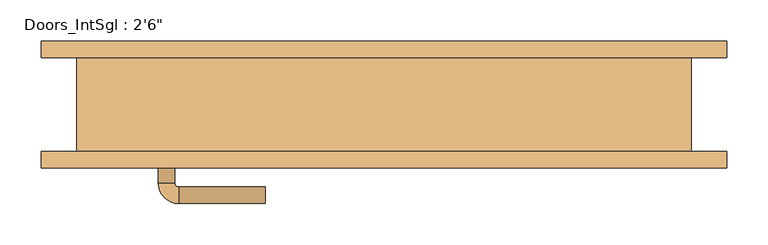
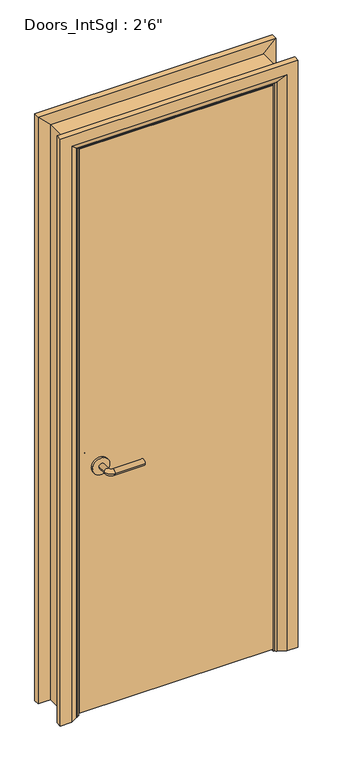
"""IFC4 building model written with IfcOpenShell, lengths in millimetres: door geometry."""

from ifc_helpers import new_model, si_unit, point, frame, frame_2d, origin, place, context, project, spatial, polyline, circle_curve, ellipse_curve, trimmed, segment, composite_curve, outline, extrude, faceted_brep, source, transform, mapped, element, save
from ifc_brep_helpers import plane_surface, cylinder_surface, revolved_surface, advanced_brep


def door_d225582b(model_context):
    return source(origin(), model_context, "Body", "SolidModel", [
        advanced_brep(
        [(-274.0, -11.15, 900.0), (-254.0, -11.15, 900.0), (-274.0, 18.85, 900.0), (-254.0, 18.85, 900.0), (-249.0, 23.85, 900.0), (-249.0, 43.85, 900.0), (-144.0, 43.85, 900.0), (-144.0, 23.85, 900.0)],
        [
            (0, 1, circle_curve(frame((-264.0, -11.15, 900.0), z_axis=(0.0, -1.0, 0.0), x_axis=(1.0, 0.0, 0.0)), 10.0)),
            (1, 0, circle_curve(frame((-264.0, -11.15, 900.0), z_axis=(0.0, -1.0, 0.0), x_axis=(1.0, 0.0, 0.0)), 10.0)),
            (0, 2),
            (2, 3, circle_curve(frame((-264.0, 18.85, 900.0), z_axis=(0.0, -1.0, 0.0), x_axis=(1.0, 0.0, 0.0)), 10.0)),
            (3, 1),
            (3, 2, circle_curve(frame((-264.0, 18.85, 900.0), z_axis=(0.0, -1.0, 0.0), x_axis=(1.0, 0.0, 0.0)), 10.0)),
            (4, 3, circle_curve(frame((-249.0, 18.85, 900.0), z_axis=(0.0, 0.0, 1.0), x_axis=(-1.0, 0.0, 0.0)), 5.0)),
            (2, 5, circle_curve(frame((-249.0, 18.85, 900.0), z_axis=(0.0, 0.0, -1.0), x_axis=(-1.0, 0.0, 0.0)), 25.0)),
            (5, 4, circle_curve(frame((-249.0, 33.85, 900.0), z_axis=(-1.0, 0.0, 0.0), x_axis=(0.0, -1.0, 0.0)), 10.0)),
            (4, 5, circle_curve(frame((-249.0, 33.85, 900.0), z_axis=(-1.0, 0.0, 0.0), x_axis=(0.0, -1.0, 0.0)), 10.0)),
            (6, 7, circle_curve(frame((-144.0, 33.85, 900.0), z_axis=(1.0, 0.0, 0.0), x_axis=(0.0, -1.0, 0.0)), 10.0)),
            (7, 6, circle_curve(frame((-144.0, 33.85, 900.0), z_axis=(1.0, 0.0, 0.0), x_axis=(0.0, -1.0, 0.0)), 10.0)),
            (5, 6),
            (7, 4),
        ],
        [
            plane_surface(frame((-264.0, -11.15, 900.0), z_axis=(0.0, -1.0, 0.0), x_axis=(0.0, 0.0, 1.0))),
            cylinder_surface(frame((-264.0, -11.15, 900.0), z_axis=(0.0, -1.0, 0.0), x_axis=(1.0, 0.0, 0.0)), 10.0),
            revolved_surface(trimmed(ellipse_curve(frame((-264.0, 18.85, 900.0), z_axis=(0.0, -1.0, 0.0), x_axis=(1.0, 0.0, 0.0)), 10.0, 10.0), [point((-274.0, 18.85, 900.0))], [point((-254.0, 18.85, 900.0))], True, "CARTESIAN"), (-249.0, 18.85, 900.0), (0.0, 0.0, -1.0)),
            revolved_surface(trimmed(ellipse_curve(frame((-264.0, 18.85, 900.0), z_axis=(0.0, -1.0, 0.0), x_axis=(1.0, 0.0, 0.0)), 10.0, 10.0), [point((-254.0, 18.85, 900.0))], [point((-274.0, 18.85, 900.0))], True, "CARTESIAN"), (-249.0, 18.85, 900.0), (0.0, 0.0, -1.0)),
            plane_surface(frame((-144.0, 33.85, 900.0), z_axis=(1.0, 0.0, 0.0), x_axis=(0.0, 0.0, 1.0))),
            cylinder_surface(frame((-249.0, 33.85, 900.0), z_axis=(-1.0, 0.0, 0.0), x_axis=(0.0, -1.0, 0.0)), 10.0),
        ],
        [
            (0, [[1, 2]]),
            (1, [[-1, 3, 4, 5]]),
            (1, [[-2, -5, 6, -3]]),
            (2, [[7, -4, 8, 9]]),
            (3, [[-8, -6, -7, 10]]),
            (4, [[11, 12]]),
            (5, [[-9, 13, -12, 14]]),
            (5, [[-10, -14, -11, -13]]),
        ],
    ),
        extrude(outline(composite_curve([segment(trimmed(circle_curve(frame_2d((900.0, -266.5)), 30.0), [point((900.0, -296.5))], [point((900.0, -236.5))], False, "CARTESIAN"), True, "CONTINUOUS"), segment(trimmed(circle_curve(frame_2d((900.0, -266.5)), 30.0), [point((900.0, -236.5))], [point((900.0, -296.5))], False, "CARTESIAN"), True, "CONTINUOUS")], self_intersect=False)), frame((0.0, -19.15, 0.0), z_axis=(0.0, 1.0, 0.0), x_axis=(0.0, 0.0, 1.0)), (0.0, 0.0, 1.0), 8.0),
        advanced_brep(
        [(-274.0, -65.15, 900.0), (-254.0, -65.15, 900.0), (-254.0, -95.15, 900.0), (-274.0, -95.15, 900.0), (-249.0, -100.15, 900.0), (-249.0, -120.15, 900.0), (-144.0, -120.15, 900.0), (-144.0, -100.15, 900.0)],
        [
            (0, 1, circle_curve(frame((-264.0, -65.15, 900.0), z_axis=(0.0, 1.0, 0.0), x_axis=(1.0, 0.0, 0.0)), 10.0)),
            (1, 0, circle_curve(frame((-264.0, -65.15, 900.0), z_axis=(0.0, 1.0, 0.0), x_axis=(1.0, 0.0, 0.0)), 10.0)),
            (1, 2),
            (2, 3, circle_curve(frame((-264.0, -95.15, 900.0), z_axis=(0.0, 1.0, 0.0), x_axis=(1.0, 0.0, 0.0)), 10.0)),
            (3, 0),
            (3, 2, circle_curve(frame((-264.0, -95.15, 900.0), z_axis=(0.0, 1.0, 0.0), x_axis=(1.0, 0.0, 0.0)), 10.0)),
            (4, 5, circle_curve(frame((-249.0, -110.15, 900.0), z_axis=(-1.0, 0.0, 0.0), x_axis=(0.0, 1.0, 0.0)), 10.0)),
            (5, 3, circle_curve(frame((-249.0, -95.15, 900.0), z_axis=(0.0, 0.0, -1.0), x_axis=(-1.0, 0.0, 0.0)), 25.0)),
            (2, 4, circle_curve(frame((-249.0, -95.15, 900.0), z_axis=(0.0, 0.0, 1.0), x_axis=(-1.0, 0.0, 0.0)), 5.0)),
            (5, 4, circle_curve(frame((-249.0, -110.15, 900.0), z_axis=(-1.0, 0.0, 0.0), x_axis=(0.0, 1.0, 0.0)), 10.0)),
            (6, 7, circle_curve(frame((-144.0, -110.15, 900.0), z_axis=(1.0, 0.0, 0.0), x_axis=(0.0, 1.0, 0.0)), 10.0)),
            (7, 6, circle_curve(frame((-144.0, -110.15, 900.0), z_axis=(1.0, 0.0, 0.0), x_axis=(0.0, 1.0, 0.0)), 10.0)),
            (4, 7),
            (6, 5),
        ],
        [
            plane_surface(frame((-264.0, -65.15, 900.0), z_axis=(0.0, 1.0, 0.0), x_axis=(0.0, 0.0, 1.0))),
            cylinder_surface(frame((-264.0, -65.15, 900.0), z_axis=(0.0, 1.0, 0.0), x_axis=(1.0, 0.0, 0.0)), 10.0),
            revolved_surface(trimmed(ellipse_curve(frame((-264.0, -95.15, 900.0), z_axis=(0.0, -1.0, 0.0), x_axis=(1.0, 0.0, 0.0)), 10.0, 10.0), [point((-274.0, -95.15, 900.0))], [point((-254.0, -95.15, 900.0))], True, "CARTESIAN"), (-249.0, -95.15, 900.0), (0.0, 0.0, -1.0)),
            revolved_surface(trimmed(ellipse_curve(frame((-264.0, -95.15, 900.0), z_axis=(0.0, -1.0, 0.0), x_axis=(1.0, 0.0, 0.0)), 10.0, 10.0), [point((-254.0, -95.15, 900.0))], [point((-274.0, -95.15, 900.0))], True, "CARTESIAN"), (-249.0, -95.15, 900.0), (0.0, 0.0, -1.0)),
            plane_surface(frame((-144.0, -110.15, 900.0), z_axis=(1.0, 0.0, 0.0), x_axis=(0.0, 0.0, 1.0))),
            cylinder_surface(frame((-249.0, -110.15, 900.0), z_axis=(-1.0, 0.0, 0.0), x_axis=(0.0, 1.0, 0.0)), 10.0),
        ],
        [
            (0, [[1, 2]]),
            (1, [[3, 4, 5, -2]]),
            (1, [[-5, 6, -3, -1]]),
            (2, [[7, 8, -4, 9]]),
            (3, [[10, -9, -6, -8]]),
            (4, [[11, 12]]),
            (5, [[13, -11, 14, -7]]),
            (5, [[-14, -12, -13, -10]]),
        ],
    ),
        extrude(outline(composite_curve([segment(trimmed(circle_curve(frame_2d((900.0, -266.5)), 30.0), [point((900.0, -296.5))], [point((900.0, -236.5))], False, "CARTESIAN"), True, "CONTINUOUS"), segment(trimmed(circle_curve(frame_2d((900.0, -266.5)), 30.0), [point((900.0, -236.5))], [point((900.0, -296.5))], False, "CARTESIAN"), True, "CONTINUOUS")], self_intersect=False)), frame((0.0, -65.15, 0.0), z_axis=(0.0, 1.0, 0.0), x_axis=(0.0, 0.0, 1.0)), (0.0, 0.0, 1.0), 8.0),
        extrude(outline(polyline([(339.0, -19.15), (339.0, -57.15), (-339.0, -57.15), (-339.0, -19.15), (339.0, -19.15)])), frame((0.0, 0.0, 8.0), z_axis=(0.0, 0.0, 1.0), x_axis=(1.0, 0.0, 0.0)), (0.0, 0.0, 1.0), 2083.6),
        advanced_brep(
        [(416.0, -77.15, 0.0), (376.0, -77.15, 0.0), (350.0, -63.15, 0.0), (346.0, -57.15, 0.0), (416.0, -57.15, 0.0), (416.0, -57.15, 2168.6), (416.0, -77.15, 2168.6), (346.0, -57.15, 2098.6), (-346.0, -57.15, 2098.6), (-346.0, -57.15, 0.0), (-416.0, -57.15, 0.0), (-416.0, -57.15, 2168.6), (350.0, -63.15, 2102.6), (376.0, -77.15, 2128.6), (-416.0, -77.15, 2168.6), (-416.0, -77.15, 0.0), (-376.0, -77.15, 0.0), (-376.0, -77.15, 2128.6), (-350.0, -63.15, 0.0), (-350.0, -63.15, 2102.6)],
        [
            (0, 1),
            (1, 2),
            (2, 3, circle_curve(frame((354.0, -56.15, 0.0), z_axis=(0.0, 0.0, -1.0), x_axis=(1.0, 0.0, 0.0)), 8.0622577)),
            (3, 4),
            (4, 0),
            (4, 5),
            (5, 6),
            (6, 0),
            (3, 7),
            (7, 8),
            (8, 9),
            (9, 10),
            (10, 11),
            (11, 5),
            (2, 12),
            (12, 7, ellipse_curve(frame((354.0, -56.15, 2106.6), z_axis=(0.7071067811865475, 0.0, -0.7071067811865475), x_axis=(-0.7071067811865474, 0.0, -0.7071067811865476)), 11.4017543, 8.0622577)),
            (1, 13),
            (13, 12),
            (6, 14),
            (14, 15),
            (15, 16),
            (16, 17),
            (17, 13),
            (10, 15),
            (14, 11),
            (9, 18, circle_curve(frame((-354.0, -56.15, 0.0), z_axis=(0.0, 0.0, -1.0), x_axis=(-1.0, 0.0, 0.0)), 8.0622577)),
            (18, 16),
            (19, 18),
            (8, 19, ellipse_curve(frame((-354.0, -56.15, 2106.6), z_axis=(-0.7071067811865475, 0.0, -0.7071067811865475), x_axis=(-0.7071067811865474, 0.0, 0.7071067811865476)), 11.4017543, 8.0622577)),
            (19, 17),
            (12, 19),
        ],
        [
            plane_surface(frame((346.0, -57.15, 0.0), z_axis=(0.0, 0.0, -1.0), x_axis=(0.0, 1.0, 0.0))),
            plane_surface(frame((416.0, -77.15, 0.0), z_axis=(1.0, 0.0, 0.0), x_axis=(0.0, 0.0, 1.0))),
            plane_surface(frame((416.0, -57.15, 0.0), z_axis=(0.0, 1.0, 0.0), x_axis=(0.0, 0.0, 1.0))),
            cylinder_surface(frame((354.0, -56.15, 0.0), z_axis=(0.0, 0.0, -1.0), x_axis=(1.0, 0.0, 0.0)), 8.0622577),
            plane_surface(frame((350.0, -63.15, 0.0), z_axis=(-0.4740998230350126, -0.880471099922178, 0.0), x_axis=(0.0, 0.0, 1.0))),
            plane_surface(frame((376.0, -77.15, 0.0), z_axis=(0.0, -1.0, 0.0), x_axis=(0.0, 0.0, 1.0))),
            plane_surface(frame((-416.0, -77.15, 2168.6), z_axis=(-1.0, 0.0, 0.0), x_axis=(0.0, 0.0, -1.0))),
            plane_surface(frame((-346.0, -57.15, 0.0), z_axis=(0.0, 0.0, -1.0), x_axis=(0.0, 1.0, 0.0))),
            cylinder_surface(frame((-354.0, -56.15, 2098.6), z_axis=(0.0, 0.0, 1.0), x_axis=(-1.0, 0.0, 0.0)), 8.0622577),
            plane_surface(frame((-350.0, -63.15, 2102.6), z_axis=(0.47409982303501824, -0.8804710999221749, 0.0), x_axis=(0.0, 0.0, -1.0))),
            plane_surface(frame((416.0, -77.15, 2168.6), z_axis=(0.0, 0.0, 1.0), x_axis=(-1.0, 0.0, 0.0))),
            cylinder_surface(frame((346.0, -56.15, 2106.6), z_axis=(1.0, 0.0, 0.0), x_axis=(0.0, 0.0, 1.0)), 8.0622577),
            plane_surface(frame((350.0, -63.15, 2102.6), z_axis=(0.0, -0.8804710999221764, -0.4740998230350154), x_axis=(-1.0, 0.0, 0.0))),
        ],
        [
            (0, [[1, 2, 3, 4, 5]]),
            (1, [[6, 7, 8, -5]]),
            (2, [[9, 10, 11, 12, 13, 14, -6, -4]]),
            (3, [[15, 16, -9, -3]]),
            (4, [[17, 18, -15, -2]]),
            (5, [[-8, 19, 20, 21, 22, 23, -17, -1]]),
            (6, [[-13, 24, -20, 25]]),
            (7, [[-24, -12, 26, 27, -21]]),
            (8, [[28, -26, -11, 29]]),
            (9, [[-22, -27, -28, 30]]),
            (10, [[-14, -25, -19, -7]]),
            (11, [[31, -29, -10, -16]]),
            (12, [[-23, -30, -31, -18]]),
        ],
    ),
        extrude(outline(polyline([(0.0, -322.0), (2074.6, -322.0), (2074.6, 322.0), (0.0, 322.0), (0.0, 341.0), (2093.6, 341.0), (2093.6, -341.0), (0.0, -341.0), (0.0, -322.0)])), frame((0.0, -17.15, 0.0), z_axis=(0.0, 1.0, 0.0), x_axis=(0.0, 0.0, 1.0)), (0.0, 0.0, 1.0), 32.0),
        advanced_brep(
        [(-416.0, 77.15, 0.0), (-376.0, 77.15, 0.0), (-350.0, 63.15, 0.0), (-346.0, 57.15, 0.0), (-416.0, 57.15, 0.0), (-416.0, 57.15, 2168.6), (-416.0, 77.15, 2168.6), (-346.0, 57.15, 2098.6), (-350.0, 63.15, 2102.6), (-376.0, 77.15, 2128.6), (416.0, 77.15, 0.0), (416.0, 57.15, 0.0), (346.0, 57.15, 0.0), (350.0, 63.15, 0.0), (376.0, 77.15, 0.0), (416.0, 77.15, 2168.6), (376.0, 77.15, 2128.6), (350.0, 63.15, 2102.6), (346.0, 57.15, 2098.6), (416.0, 57.15, 2168.6)],
        [
            (0, 1),
            (1, 2),
            (2, 3, circle_curve(frame((-354.0, 56.15, 0.0), z_axis=(0.0, 0.0, -1.0), x_axis=(-1.0, 0.0, 0.0)), 8.0622577)),
            (3, 4),
            (4, 0),
            (4, 5),
            (5, 6),
            (6, 0),
            (3, 7),
            (7, 5),
            (2, 8),
            (8, 7, ellipse_curve(frame((-354.0, 56.15, 2106.6), z_axis=(-0.7071067811865475, 0.0, -0.7071067811865475), x_axis=(0.7071067811865474, 0.0, -0.7071067811865476)), 11.4017543, 8.0622577)),
            (1, 9),
            (9, 8),
            (6, 9),
            (10, 11),
            (11, 12),
            (12, 13, circle_curve(frame((354.0, 56.15, 0.0), z_axis=(0.0, 0.0, -1.0), x_axis=(1.0, 0.0, 0.0)), 8.0622577)),
            (13, 14),
            (14, 10),
            (15, 10),
            (14, 16),
            (16, 15),
            (13, 17),
            (17, 16),
            (12, 18),
            (18, 17, ellipse_curve(frame((354.0, 56.15, 2106.6), z_axis=(0.7071067811865475, 0.0, -0.7071067811865475), x_axis=(0.7071067811865474, 0.0, 0.7071067811865476)), 11.4017543, 8.0622577)),
            (11, 19),
            (19, 18),
            (15, 19),
            (5, 19),
            (15, 6),
            (7, 18),
            (8, 17),
            (9, 16),
        ],
        [
            plane_surface(frame((-346.0, 129.9510989, 0.0), z_axis=(0.0, 0.0, -1.0), x_axis=(1.0, 0.0, 0.0))),
            plane_surface(frame((-416.0, 77.15, 0.0), z_axis=(-1.0, 0.0, 0.0), x_axis=(0.0, 0.0, 1.0))),
            plane_surface(frame((-416.0, 57.15, 0.0), z_axis=(0.0, -1.0, 0.0), x_axis=(0.0, 0.0, 1.0))),
            cylinder_surface(frame((-354.0, 56.15, 0.0), z_axis=(0.0, 0.0, -1.0), x_axis=(-1.0, 0.0, 0.0)), 8.0622577),
            plane_surface(frame((-350.0, 63.15, 0.0), z_axis=(0.4740998230350183, 0.8804710999221749, 0.0), x_axis=(0.0, 0.0, 1.0))),
            plane_surface(frame((-376.0, 77.15, 0.0), z_axis=(0.0, 1.0, 0.0), x_axis=(0.0, 0.0, 1.0))),
            plane_surface(frame((346.0, 129.9510989, 0.0), z_axis=(0.0, 0.0, -1.0), x_axis=(-1.0, 0.0, 0.0))),
            plane_surface(frame((376.0, 77.15, 2128.6), z_axis=(0.0, 1.0, 0.0), x_axis=(0.0, 0.0, -1.0))),
            plane_surface(frame((350.0, 63.15, 2102.6), z_axis=(-0.4740998230350183, 0.8804710999221749, 0.0), x_axis=(0.0, 0.0, -1.0))),
            cylinder_surface(frame((354.0, 56.15, 2098.6), z_axis=(0.0, 0.0, 1.0), x_axis=(1.0, 0.0, 0.0)), 8.0622577),
            plane_surface(frame((416.0, 57.15, 2168.6), z_axis=(0.0, -1.0, 0.0), x_axis=(0.0, 0.0, -1.0))),
            plane_surface(frame((416.0, 77.15, 2168.6), z_axis=(1.0, 0.0, 0.0), x_axis=(0.0, 0.0, -1.0))),
            plane_surface(frame((-416.0, 77.15, 2168.6), z_axis=(0.0, 0.0, 1.0), x_axis=(1.0, 0.0, 0.0))),
            plane_surface(frame((-416.0, 57.15, 2168.6), z_axis=(0.0, -1.0, 0.0), x_axis=(1.0, 0.0, 0.0))),
            cylinder_surface(frame((-346.0, 56.15, 2106.6), z_axis=(-1.0, 0.0, 0.0), x_axis=(0.0, 0.0, 1.0)), 8.0622577),
            plane_surface(frame((-350.0, 63.15, 2102.6), z_axis=(0.0, 0.8804710999221749, -0.4740998230350183), x_axis=(1.0, 0.0, 0.0))),
            plane_surface(frame((-376.0, 77.15, 2128.6), z_axis=(0.0, 1.0, 0.0), x_axis=(1.0, 0.0, 0.0))),
        ],
        [
            (0, [[1, 2, 3, 4, 5]]),
            (1, [[6, 7, 8, -5]]),
            (2, [[9, 10, -6, -4]]),
            (3, [[11, 12, -9, -3]]),
            (4, [[13, 14, -11, -2]]),
            (5, [[-8, 15, -13, -1]]),
            (6, [[16, 17, 18, 19, 20]]),
            (7, [[21, -20, 22, 23]]),
            (8, [[-22, -19, 24, 25]]),
            (9, [[-24, -18, 26, 27]]),
            (10, [[-26, -17, 28, 29]]),
            (11, [[-28, -16, -21, 30]]),
            (12, [[31, -30, 32, -7]]),
            (13, [[33, -29, -31, -10]]),
            (14, [[34, -27, -33, -12]]),
            (15, [[35, -25, -34, -14]]),
            (16, [[-32, -23, -35, -15]]),
        ],
    ),
        faceted_brep([(-341.0, -57.15, 0.0), (-373.0, -57.15, 0.0), (-373.0, 57.15, 0.0), (-341.0, 57.15, 0.0), (-341.0, 57.15, 2093.6), (-341.0, -57.15, 2093.6), (-373.0, 57.15, 2125.6), (-373.0, -57.15, 2125.6), (341.0, -57.15, 0.0), (341.0, 57.15, 0.0), (373.0, 57.15, 0.0), (373.0, -57.15, 0.0), (341.0, -57.15, 2093.6), (373.0, -57.15, 2125.6), (373.0, 57.15, 2125.6), (341.0, 57.15, 2093.6)], [[[0, 1, 2, 3]], [[3, 4, 5, 0]], [[2, 6, 4, 3]], [[1, 7, 6, 2]], [[0, 5, 7, 1]], [[8, 9, 10, 11]], [[12, 8, 11, 13]], [[13, 11, 10, 14]], [[14, 10, 9, 15]], [[15, 9, 8, 12]], [[4, 15, 12, 5]], [[6, 14, 15, 4]], [[7, 13, 14, 6]], [[5, 12, 13, 7]]]),
    ])


if __name__ == "__main__":
    model = new_model("IFC4")
    model_context = context("Model", 3, world=origin())
    ifc_project = project(units=[si_unit("LENGTHUNIT", "METRE", prefix="MILLI")], contexts=[model_context])
    site = spatial("IfcSite", under=ifc_project)
    building = spatial("IfcBuilding", under=site)
    placement = place(None, origin())
    door_shape = door_d225582b(model_context)
    element("IfcDoor", 1, ObjectType="Doors_IntSgl : 2'6\"", at=placement, inside=building, context=model_context, shape_type="MappedRepresentation", body=[
        mapped(door_shape, transform((0.0, 0.0, 0.0), x_axis=(1.0, 0.0, 0.0), y_axis=(0.0, 1.0, 0.0), z_axis=(0.0, 0.0, 1.0))),
    ])
    save(model, "model.ifc")

# Revit data of these elements
# Type "Doors_IntSgl : 2'6\""
#   Type Mark = "48"
#   Type Comments = "Internal Single"
#   Operation = "SingleSwingRight"
#   Manufacturer = "Revit"
#   Keynote = "L20"
#   Description = "Internal Single Door"
#   Analytic Construction = "Metal"
#   UnderCut = 0' - 0.31496"
#   Tolerance = 0' - 0.07874"
#   Thickness = 0' - 1.49606"
#   Thermal Resistance (R) = 0.270117 (m²·K)/W
#   Structural Tolerance = 0' - 0.31496"
#   StopDepth = 0' - 1.25984"
#   Stop Thickness = 0' - 0.74803"
#   Rough Width = 2' - 6"
#   Rough Height = 7' - 0"
#   Height to Top Lock Rail = 3' - 3.37008"
#   Heat Transfer Coefficient (U) = 3.7021 W/(m²·K)
#   Handle Z Distance = 2' - 11.43307"
#   Handle X Distance = 0' - 2.95276"
#   Frame Thickness = 0' - 1.25984"
#   Door Panel Width = 2' - 2.69291"
#   Door Panel Thickness = 0' - 1.49606"
#   Door Panel Offset = 0' - 0"
#   Height = 7' - 0"
#   Width = 2' - 6"
#   Door Panel Height = 6' - 10.0315"
#   Architrave Setback = 0' - 0.19685"
#   Vis - Ironmongery = yes
#   Material Ironmongery = Door - Handle
#   Material Frame = Door - Frame/Mullion (1)
#   Material Door = Door - Panel
#   Material Architrave = Door - Architrave
#   Visual Light Transmittance = 0
#   Solar Heat Gain Coefficient = 0
#   Function = (empty or 0)
#   Wall Closure = (empty or 0)
# Element 1 (IfcDoor, "Doors_IntSgl : 2'6\"")
#   Materials on its faces: "Door - Architrave", "Door - Handle", "Door - Frame/Mullion (1)", "Door - Panel"
# Materials
#   "Door - Handle": colour RGB 0 0 0, transparency 0, Keynote = "P21", Cost = 0
#   "Door - Frame/Mullion (1)": class "Wood", colour RGB 212 179 113, transparency 0, Keynote = "L20", Cost = 0
#   "Door - Panel": class "Wood", colour RGB 210 159 95, transparency 0, Keynote = "L20", Cost = 0
#   "Door - Architrave": class "Wood", colour RGB 154 90 5, transparency 0, Keynote = "P20", Cost = 0
